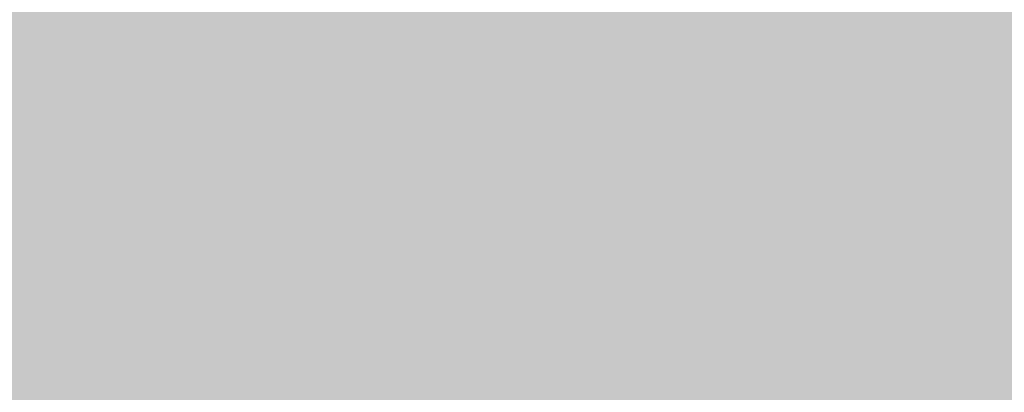
# Model space of a CAD drawing. Units: millimetres. Extents: x 0 to 2267, y 0 to 1823.
# Tile 47 of 256: x 1594.2193 to 1595.0978, y 1226.3857 to 1226.718. Entities that reach past the tile are written whole.
import ezdxf

# ---------------------------------------------------------------- set-up
doc = ezdxf.new("R2010")
doc.units = ezdxf.units.MM
doc.header["$MEASUREMENT"] = 0
doc.layers.add('M-HATC', color=252, linetype='Continuous', lineweight=18)

msp = doc.modelspace()

# ---------------------------------------------------------------- hatches: boundary and pattern name
at = {"layer": 'M-HATC'}
h = msp.add_hatch(color=256, dxfattribs=at)
h.dxf.hatch_style = 1
h.paths.add_polyline_path([(2055.77105, 1603.06204), (1381.08677, 1603.06204), (1381.08677, 1598.06204), (2055.77105, 1598.06204)])
h.paths.add_polyline_path([(2055.77105, 1598.06204), (1381.08677, 1598.06204), (1381.08677, 1593.06204), (2055.77105, 1593.06204)])
h.paths.add_polyline_path([(2051.30737, 1536.76088), (1385.55044, 1536.76088), (1385.55044, 1526.76088), (1387.55044, 1526.76088), (1388.53662, 1525.05276), (1385.33187, 1521.23348), (1385.33187, 1521.22256), (2050.25417, 1522.74913), (2048.32119, 1525.05276), (2049.30737, 1526.76088), (2051.30737, 1526.76088)])
edge = h.paths.add_edge_path()
edge.add_arc((1847.53451, 1379.14917), 135, 222.6030607, 222.8908505, ccw=False)
edge.add_line((1748.16629, 1287.76561), (1683.09212, 1287.76561))
edge.add_arc((1583.7239, 1379.14917), 135, 317.1091495, 317.3969393, ccw=False)
edge.add_arc((1678.9686, 1290.67067), 5, 222.89085, 317.10915, ccw=False)
edge.add_arc((1774.21331, 1379.14917), 135, 222.6030607, 222.8908505, ccw=False)
edge.add_line((1674.84509, 1287.76561), (1609.77092, 1287.76561))
edge.add_arc((1510.4027, 1379.14917), 135, 317.1091495, 317.3969393, ccw=False)
edge.add_arc((1605.6474, 1290.67067), 5, 222.89085, 317.10915, ccw=False)
edge.add_arc((1700.89211, 1379.14917), 135, 222.6030607, 222.8908505, ccw=False)
edge.add_line((1601.52388, 1287.76561), (1536.44972, 1287.76561))
edge.add_arc((1437.08149, 1379.14917), 135, 317.1091495, 317.3969393, ccw=False)
edge.add_arc((1532.3262, 1290.67067), 5, 222.89085, 317.10915, ccw=False)
edge.add_arc((1627.57091, 1379.14917), 135, 222.6030607, 222.8908505, ccw=False)
edge.add_line((1528.20268, 1287.76561), (1505.92891, 1287.76561))
edge.add_spline(control_points=[(1505.92891, 1287.76561), (1504.26224, 1287.76561), (1504.26224, 1282.76561), (1505.92891, 1282.76561)], knot_values=[0, 0, 0, 0, 5, 5, 5, 5], degree=3, periodic=0)
edge.add_line((1505.92891, 1282.76561), (1930.92891, 1282.76561))
edge.add_spline(control_points=[(1930.92891, 1282.76561), (1932.59557, 1282.76561), (1932.59557, 1287.76561), (1930.92891, 1287.76561)], knot_values=[0, 0, 0, 0, 5, 5, 5, 5], degree=3, periodic=0)
edge.add_line((1930.92891, 1287.76561), (1903.05573, 1287.76561))
edge.add_arc((1803.6875, 1379.14917), 135, 317.1091495, 317.3969393, ccw=False)
edge.add_arc((1898.93221, 1290.67067), 5, 222.89085, 317.10915, ccw=False)
edge.add_arc((1994.17691, 1379.14917), 135, 222.6030607, 222.8908505, ccw=False)
edge.add_line((1894.80869, 1287.76561), (1829.73452, 1287.76561))
edge.add_arc((1730.3663, 1379.14917), 135, 317.1091495, 317.3969393, ccw=False)
edge.add_arc((1825.61101, 1290.67067), 5, 222.89085, 317.10915, ccw=False)
edge.add_arc((1920.85571, 1379.14917), 135, 222.6030607, 222.8908505, ccw=False)
edge.add_line((1821.48749, 1287.76561), (1756.41332, 1287.76561))
edge.add_arc((1657.0451, 1379.14917), 135, 317.1091495, 317.3969393, ccw=False)
edge.add_arc((1752.28981, 1290.67067), 5, 222.89085, 317.10915, ccw=False)
edge = h.paths.add_edge_path()
edge.add_spline(control_points=[(1843.42891, 1227.24746), (1845.09557, 1227.24746), (1845.09557, 1232.24746), (1843.42891, 1232.24746)], knot_values=[0, 0, 0, 0, 5, 5, 5, 5], degree=3, periodic=0)
edge.add_line((1843.42891, 1232.24746), (1593.42891, 1232.24746))
edge.add_spline(control_points=[(1593.42891, 1232.24746), (1591.76224, 1232.24746), (1591.76224, 1227.24746), (1593.42891, 1227.24746)], knot_values=[0, 0, 0, 0, 5, 5, 5, 5], degree=3, periodic=0)
edge.add_line((1593.42891, 1227.24746), (1843.42891, 1227.24746))
h.paths.add_polyline_path([(1905.92891, 1127.41706), (1530.92891, 1127.41706, 0.414214), (1520.92891, 1117.41706), (1530.92891, 1117.41706), (1915.92891, 1117.41706, 0.414214)])
edge = h.paths.add_edge_path()
edge.add_arc((1397.08577, 1498.40775), 12.72993, 90.782146, 190.878706, ccw=False)
edge.add_line((1396.912, 1511.13649), (1428.00968, 1511.34875))
edge.add_line((1428.00968, 1511.34875), (1433.00968, 1511.34875))
edge.add_line((1433.00968, 1511.34875), (1434.439, 1511.34875))
edge.add_arc((1419.474, 1498.08041), 20, 41.560995, 74.082109)
edge.add_line((1424.95919, 1517.31353), (1399.93509, 1517.25608))
edge.add_spline(control_points=[(1399.93074, 1517.25607), (1399.88398, 1517.21312), (1399.8328, 1517.16893), (1399.77741, 1517.1236)], knot_values=[11.567499, 11.567499, 11.567499, 11.567499, 11.814249, 11.814249, 11.814249, 11.814249], degree=3, periodic=0)
edge.add_spline(control_points=[(1399.63279, 1517.00986), (1399.58305, 1516.97214), (1399.53072, 1516.93375), (1399.47591, 1516.89474)], knot_values=[11.167718, 11.167718, 11.167718, 11.167718, 11.365188, 11.365188, 11.365188, 11.365188], degree=3, periodic=0)
edge.add_spline(control_points=[(1399.33981, 1516.80007), (1399.15144, 1516.67185), (1398.93836, 1516.5377), (1398.70404, 1516.39942)], knot_values=[10.376405, 10.376405, 10.376405, 10.376405, 11.00994, 11.00994, 11.00994, 11.00994], degree=3, periodic=0)
edge.add_spline(control_points=[(1398.65716, 1516.37187), (1398.57885, 1516.32602), (1398.49825, 1516.27974), (1398.41549, 1516.23309)], knot_values=[10.125175, 10.125175, 10.125175, 10.125175, 10.334406, 10.334406, 10.334406, 10.334406], degree=3, periodic=0)
edge.add_spline(control_points=[(1398.26422, 1516.14874), (1398.19595, 1516.11107), (1398.12634, 1516.07319), (1398.05546, 1516.03513)], knot_values=[9.832246, 9.832246, 9.832246, 9.832246, 9.999658, 9.999658, 9.999658, 9.999658], degree=3, periodic=0)
edge.add_spline(control_points=[(1397.9987, 1516.00476), (1397.73115, 1515.86211), (1397.44602, 1515.71707), (1397.14664, 1515.57138)], knot_values=[9.161808, 9.161808, 9.161808, 9.161808, 9.787769, 9.787769, 9.787769, 9.787769], degree=3, periodic=0)
edge.add_spline(control_points=[(1397.14664, 1515.57138), (1396.84182, 1515.42305), (1396.52223, 1515.27404), (1396.1914, 1515.12621)], knot_values=[8.524455, 8.524455, 8.524455, 8.524455, 9.161808, 9.161808, 9.161808, 9.161808], degree=3, periodic=0)
edge.add_spline(control_points=[(1396.07771, 1515.07565), (1395.98538, 1515.03478), (1395.89222, 1514.99402), (1395.7983, 1514.9534)], knot_values=[8.275193, 8.275193, 8.275193, 8.275193, 8.451726, 8.451726, 8.451726, 8.451726], degree=3, periodic=0)
edge.add_spline(control_points=[(1395.60184, 1514.86912), (1395.49975, 1514.82568), (1395.39685, 1514.78244), (1395.29322, 1514.73944)], knot_values=[7.962917, 7.962917, 7.962917, 7.962917, 8.152764, 8.152764, 8.152764, 8.152764], degree=3, periodic=0)
edge.add_spline(control_points=[(1395.21158, 1514.70568), (1394.82779, 1514.5475), (1394.43452, 1514.39287), (1394.03645, 1514.24422)], knot_values=[7.21254, 7.21254, 7.21254, 7.21254, 7.913148, 7.913148, 7.913148, 7.913148], degree=3, periodic=0)
edge.add_spline(control_points=[(1394.03645, 1514.24422), (1393.70758, 1514.12142), (1393.37544, 1514.0027), (1393.04267, 1513.88945)], knot_values=[6.633733, 6.633733, 6.633733, 6.633733, 7.21254, 7.21254, 7.21254, 7.21254], degree=3, periodic=0)
edge.add_spline(control_points=[(1392.82142, 1513.81499), (1392.71978, 1513.78118), (1392.61815, 1513.74791), (1392.51658, 1513.71521)], knot_values=[6.328796, 6.328796, 6.328796, 6.328796, 6.505493, 6.505493, 6.505493, 6.505493], degree=3, periodic=0)
edge.add_spline(control_points=[(1392.51658, 1513.71521), (1392.31873, 1513.65151), (1392.12116, 1513.59001), (1391.92441, 1513.53098)], knot_values=[5.984605, 5.984605, 5.984605, 5.984605, 6.328796, 6.328796, 6.328796, 6.328796], degree=3, periodic=0)
edge.add_spline(control_points=[(1391.79155, 1513.49146), (1391.31215, 1513.35011), (1390.83842, 1513.22392), (1390.37844, 1513.11711)], knot_values=[5.066697, 5.066697, 5.066697, 5.066697, 5.907055, 5.907055, 5.907055, 5.907055], degree=3, periodic=0)
edge.add_spline(control_points=[(1390.37844, 1513.11711), (1390.17973, 1513.07097), (1389.98359, 1513.02845), (1389.79067, 1512.98988)], knot_values=[4.70367, 4.70367, 4.70367, 4.70367, 5.066695, 5.066695, 5.066695, 5.066695], degree=3, periodic=0)
edge.add_spline(control_points=[(1389.42203, 1512.92036), (1389.24588, 1512.88922), (1389.0729, 1512.86172), (1388.90364, 1512.83814)], knot_values=[4.130571, 4.130571, 4.130571, 4.130571, 4.469816, 4.469816, 4.469816, 4.469816], degree=3, periodic=0)
edge.add_spline(control_points=[(1388.90364, 1512.83814), (1388.59103, 1512.7946), (1388.29108, 1512.76444), (1388.00714, 1512.74941)], knot_values=[3.504031, 3.504031, 3.504031, 3.504031, 4.130571, 4.130571, 4.130571, 4.130571], degree=3, periodic=0)
edge.add_spline(control_points=[(1387.9356, 1512.74593), (1387.85378, 1512.74231), (1387.77334, 1512.73997), (1387.69435, 1512.73898)], knot_values=[3.268866, 3.268866, 3.268866, 3.268866, 3.451164, 3.451164, 3.451164, 3.451164], degree=3, periodic=0)
edge.add_spline(control_points=[(1387.33512, 1512.74426), (1387.20757, 1512.74991), (1387.08472, 1512.7597), (1386.96699, 1512.77385)], knot_values=[2.670686, 2.670686, 2.670686, 2.670686, 2.984, 2.984, 2.984, 2.984], degree=3, periodic=0)
edge.add_spline(control_points=[(1386.83274, 1512.79225), (1386.82093, 1512.79407), (1386.80917, 1512.79594), (1386.79747, 1512.79787)], knot_values=[2.516981, 2.516981, 2.516981, 2.516981, 2.549528, 2.549528, 2.549528, 2.549528], degree=3, periodic=0)
edge.add_spline(control_points=[(1386.45257, 1512.87348), (1386.42573, 1512.88105), (1386.39931, 1512.88895), (1386.3733, 1512.89719)], knot_values=[2.095869, 2.095869, 2.095869, 2.095869, 2.17941, 2.17941, 2.17941, 2.17941], degree=3, periodic=0)
edge.add_spline(control_points=[(1386.06911, 1513.01889), (1386.06338, 1513.02174), (1386.05768, 1513.02463), (1386.05201, 1513.02753)], knot_values=[1.72453, 1.72453, 1.72453, 1.72453, 1.745933, 1.745933, 1.745933, 1.745933], degree=3, periodic=0)
edge.add_arc((1399.474, 1498.08041), 20, 131.824322, 180)
edge.add_arc((1630.33362, 1505.54843), 250.97076, 181.7051759, 236.427975)
edge.add_arc((1605.33992, 1483.30441), 218.7822, 238.660829, 243.3496099)
edge.add_arc((1647.09105, 1510.35917), 262.89859, 183.1298361, 237.8534422, ccw=False)
h.paths.add_polyline_path([(1406.53685, 1391.96444, 0.149382), (1491.55061, 1296.44177, -0.129517)], flags=17)
edge = h.paths.add_edge_path()
edge.add_arc((2037.38381, 1498.08041), 20, 0, 48.265868)
edge.add_spline(control_points=[(2050.69731, 1513.00525), (2050.65121, 1512.98471), (2050.60338, 1512.96554), (2050.55388, 1512.94771)], knot_values=[1.835652, 1.835652, 1.835652, 1.835652, 2.000781, 2.000781, 2.000781, 2.000781], degree=3, periodic=0)
edge.add_spline(control_points=[(2050.46156, 1512.91661), (2050.479, 1512.9221), (2050.49625, 1512.92774), (2050.51332, 1512.93353)], knot_values=[2.045477, 2.045477, 2.045477, 2.045477, 2.101389, 2.101389, 2.101389, 2.101389], degree=3, periodic=0)
edge.add_spline(control_points=[(2050.12896, 1512.83416), (2050.19843, 1512.84734), (2050.26573, 1512.86233), (2050.33075, 1512.87919)], knot_values=[2.237629, 2.237629, 2.237629, 2.237629, 2.435841, 2.435841, 2.435841, 2.435841], degree=3, periodic=0)
edge.add_spline(control_points=[(2050.09463, 1512.82783), (2050.10613, 1512.82989), (2050.11757, 1512.832), (2050.12896, 1512.83416)], knot_values=[2.435841, 2.435841, 2.435841, 2.435841, 2.468321, 2.468321, 2.468321, 2.468321], degree=3, periodic=0)
edge.add_spline(control_points=[(2049.78433, 1512.78511), (2049.85521, 1512.79219), (2049.92435, 1512.80077), (2049.99166, 1512.81088)], knot_values=[2.563852, 2.563852, 2.563852, 2.563852, 2.748541, 2.748541, 2.748541, 2.748541], degree=3, periodic=0)
edge.add_spline(control_points=[(2049.4052, 1512.76169), (2049.5364, 1512.76526), (2049.66292, 1512.77299), (2049.78433, 1512.78511)], knot_values=[2.748541, 2.748541, 2.748541, 2.748541, 3.064882, 3.064882, 3.064882, 3.064882], degree=3, periodic=0)
edge.add_spline(control_points=[(2049.16976, 1512.75968), (2049.23364, 1512.7591), (2049.29654, 1512.7594), (2049.35844, 1512.7606)], knot_values=[3.102309, 3.102309, 3.102309, 3.102309, 3.2503, 3.2503, 3.2503, 3.2503], degree=3, periodic=0)
edge.add_spline(control_points=[(2048.85727, 1512.76911), (2048.96378, 1512.76378), (2049.068, 1512.76061), (2049.16976, 1512.75968)], knot_values=[3.2503, 3.2503, 3.2503, 3.2503, 3.486069, 3.486069, 3.486069, 3.486069], degree=3, periodic=0)
edge.add_spline(control_points=[(2048.69241, 1512.77892), (2048.3729, 1512.80093), (2048.0345, 1512.84106), (2047.68175, 1512.89697)], knot_values=[3.606429, 3.606429, 3.606429, 3.606429, 4.2989, 4.2989, 4.2989, 4.2989], degree=3, periodic=0)
edge.add_spline(control_points=[(2047.68175, 1512.89697), (2047.5458, 1512.91852), (2047.40772, 1512.94241), (2047.26776, 1512.96851)], knot_values=[4.2989, 4.2989, 4.2989, 4.2989, 4.565769, 4.565769, 4.565769, 4.565769], degree=3, periodic=0)
edge.add_spline(control_points=[(2047.26776, 1512.96851), (2047.14494, 1512.99141), (2047.02067, 1513.01601), (2046.89514, 1513.04223)], knot_values=[4.565769, 4.565769, 4.565769, 4.565769, 4.799971, 4.799971, 4.799971, 4.799971], degree=3, periodic=0)
edge.add_spline(control_points=[(2046.89514, 1513.04223), (2046.52865, 1513.11875), (2046.15135, 1513.20899), (2045.7676, 1513.31068)], knot_values=[4.799971, 4.799971, 4.799971, 4.799971, 5.483718, 5.483718, 5.483718, 5.483718], degree=3, periodic=0)
edge.add_spline(control_points=[(2045.7676, 1513.31068), (2045.3724, 1513.41539), (2044.97036, 1513.53225), (2044.56625, 1513.65876)], knot_values=[5.483718, 5.483718, 5.483718, 5.483718, 6.187866, 6.187866, 6.187866, 6.187866], degree=3, periodic=0)
edge.add_spline(control_points=[(2044.56625, 1513.65876), (2044.41491, 1513.70614), (2044.26329, 1513.75487), (2044.11163, 1513.80482)], knot_values=[6.187866, 6.187866, 6.187866, 6.187866, 6.451551, 6.451551, 6.451551, 6.451551], degree=3, periodic=0)
edge.add_spline(control_points=[(2044.11163, 1513.80482), (2043.99666, 1513.84269), (2043.88167, 1513.88126), (2043.76676, 1513.92048)], knot_values=[6.451551, 6.451551, 6.451551, 6.451551, 6.651434, 6.651434, 6.651434, 6.651434], degree=3, periodic=0)
edge.add_spline(control_points=[(2043.76676, 1513.92048), (2043.37157, 1514.05536), (2042.97738, 1514.19789), (2042.58863, 1514.34575)], knot_values=[6.651434, 6.651434, 6.651434, 6.651434, 7.338879, 7.338879, 7.338879, 7.338879], degree=3, periodic=0)
edge.add_spline(control_points=[(2042.58863, 1514.34575), (2042.16431, 1514.50715), (2041.74647, 1514.67491), (2041.34086, 1514.84603)], knot_values=[7.338879, 7.338879, 7.338879, 7.338879, 8.089209, 8.089209, 8.089209, 8.089209], degree=3, periodic=0)
edge.add_spline(control_points=[(2041.34086, 1514.84603), (2041.1028, 1514.94647), (2040.86896, 1515.04806), (2040.64049, 1515.1502)], knot_values=[8.089209, 8.089209, 8.089209, 8.089209, 8.529587, 8.529587, 8.529587, 8.529587], degree=3, periodic=0)
edge.add_spline(control_points=[(2040.50999, 1515.20887), (2040.08238, 1515.40218), (2039.67475, 1515.59705), (2039.29495, 1515.78939)], knot_values=[8.613818, 8.613818, 8.613818, 8.613818, 9.44571, 9.44571, 9.44571, 9.44571], degree=3, periodic=0)
edge.add_spline(control_points=[(2039.29495, 1515.78939), (2039.0618, 1515.90746), (2038.83914, 1516.02458), (2038.62878, 1516.1398)], knot_values=[9.44571, 9.44571, 9.44571, 9.44571, 9.956404, 9.956404, 9.956404, 9.956404], degree=3, periodic=0)
edge.add_spline(control_points=[(2038.62878, 1516.1398), (2038.51874, 1516.20007), (2038.41207, 1516.25982), (2038.30903, 1516.31891)], knot_values=[9.956404, 9.956404, 9.956404, 9.956404, 10.223542, 10.223542, 10.223542, 10.223542], degree=3, periodic=0)
edge.add_spline(control_points=[(2038.30903, 1516.31891), (2038.21377, 1516.37354), (2038.12161, 1516.42762), (2038.03275, 1516.48102)], knot_values=[10.223542, 10.223542, 10.223542, 10.223542, 10.47051, 10.47051, 10.47051, 10.47051], degree=3, periodic=0)
edge.add_spline(control_points=[(2038.03275, 1516.48102), (2037.78552, 1516.62961), (2037.56388, 1516.77304), (2037.37225, 1516.909)], knot_values=[10.47051, 10.47051, 10.47051, 10.47051, 11.15767, 11.15767, 11.15767, 11.15767], degree=3, periodic=0)
edge.add_spline(control_points=[(2037.37225, 1516.909), (2037.27893, 1516.9752), (2037.19274, 1517.03963), (2037.11417, 1517.10203)], knot_values=[11.15767, 11.15767, 11.15767, 11.15767, 11.49227, 11.49227, 11.49227, 11.49227], degree=3, periodic=0)
edge.add_spline(control_points=[(2036.85638, 1517.32585), (2036.91481, 1517.26923), (2036.98143, 1517.21027), (2037.05573, 1517.14922)], knot_values=[11.577341, 11.577341, 11.577341, 11.577341, 11.91035, 11.91035, 11.91035, 11.91035], degree=3, periodic=0)
edge.add_spline(control_points=[(2036.80739, 1517.37475), (2036.82301, 1517.35865), (2036.83935, 1517.34235), (2036.85638, 1517.32585)], knot_values=[11.91035, 11.91035, 11.91035, 11.91035, 12.007402, 12.007402, 12.007402, 12.007402], degree=3, periodic=0)
edge.add_spline(control_points=[(2036.70167, 1517.494), (2036.71042, 1517.48299), (2036.71958, 1517.47185), (2036.72913, 1517.4606)], knot_values=[12.184155, 12.184155, 12.184155, 12.184155, 12.255409, 12.255409, 12.255409, 12.255409], degree=3, periodic=0)
edge.add_spline(control_points=[(2036.6159, 1517.6205), (2036.61998, 1517.61304), (2036.6243, 1517.6055), (2036.62885, 1517.59789)], knot_values=[12.487913, 12.487913, 12.487913, 12.487913, 12.541035, 12.541035, 12.541035, 12.541035], degree=3, periodic=0)
edge.add_spline(control_points=[(2036.56349, 1517.78599), (2036.56372, 1517.77936), (2036.56423, 1517.77264), (2036.56502, 1517.76582)], knot_values=[12.911761, 12.911761, 12.911761, 12.911761, 12.968286, 12.968286, 12.968286, 12.968286], degree=3, periodic=0)
edge.add_spline(control_points=[(2036.61663, 1517.93042), (2036.61248, 1517.92586), (2036.60857, 1517.92121), (2036.60491, 1517.91648)], knot_values=[13.382527, 13.382527, 13.382527, 13.382527, 13.433791, 13.433791, 13.433791, 13.433791], degree=3, periodic=0)
edge.add_spline(control_points=[(2036.74902, 1518.01695), (2036.73613, 1518.0116), (2036.72393, 1518.00601), (2036.71242, 1518.00018)], knot_values=[13.726299, 13.726299, 13.726299, 13.726299, 13.809928, 13.809928, 13.809928, 13.809928], degree=3, periodic=0)
edge.add_spline(control_points=[(2036.86043, 1518.05285), (2036.83863, 1518.04743), (2036.81809, 1518.04156), (2036.79879, 1518.03526)], knot_values=[13.910887, 13.910887, 13.910887, 13.910887, 14.02153, 14.02153, 14.02153, 14.02153], degree=3, periodic=0)
edge.add_line((2036.96387, 1518.08041), (2032.38381, 1518.08041))
edge.add_line((2032.38381, 1518.08041), (2027.38381, 1518.08041))
edge.add_line((2027.38381, 1518.08041), (2022.38381, 1518.08041))
edge.add_line((2022.38381, 1518.08041), (2017.38381, 1518.08041))
edge.add_arc((2017.38381, 1498.08041), 20, 90, 138.439005)
edge.add_line((2002.41881, 1511.34875), (2003.84813, 1511.34875))
edge.add_line((2003.84813, 1511.34875), (2008.84813, 1511.34875))
edge.add_line((2008.84813, 1511.34875), (2039.77204, 1511.13768))
edge.add_arc((2039.77204, 1498.40775), 12.72993, -10.878706, 90, ccw=False)
edge.add_arc((1789.76676, 1510.35917), 262.89859, 302.1465578, 356.8701639, ccw=False)
edge.add_arc((1831.51789, 1483.30441), 218.7822, 296.6503901, 301.339171)
edge.add_arc((1806.52419, 1505.54843), 250.97076, 303.572025, 358.2948241)
h.paths.add_polyline_path([(2030.32096, 1391.96444, -0.129517), (1945.3072, 1296.44177, 0.149382)], flags=17)
edge = h.paths.add_edge_path()
edge.add_spline(control_points=[(2037.2464, 1518.08209), (2037.28977, 1518.08098), (2037.33555, 1518.08041), (2037.3838, 1518.08041)], knot_values=[0.000012, 0.000012, 0.000012, 0.000012, 0.144754, 0.144754, 0.144754, 0.144754], degree=3, periodic=0)
edge.add_line((2037.33571, 1518.08041), (2037.00963, 1518.08041))
edge.add_spline(control_points=[(2037.00963, 1518.08041), (2036.98217, 1518.07678), (2036.95605, 1518.07266), (2036.93124, 1518.06808)], knot_values=[14.13465, 14.13465, 14.13465, 14.13465, 14.247197, 14.247197, 14.247197, 14.247197], degree=3, periodic=0)
edge.add_spline(control_points=[(2036.93124, 1518.06808), (2036.92764, 1518.06741), (2036.92407, 1518.06674), (2036.92053, 1518.06605)], knot_values=[14.118315, 14.118315, 14.118315, 14.118315, 14.13465, 14.13465, 14.13465, 14.13465], degree=3, periodic=0)
edge.add_spline(control_points=[(2036.92053, 1518.06605), (2036.9118, 1518.06436), (2036.90323, 1518.06262), (2036.89484, 1518.06081)], knot_values=[14.078086, 14.078086, 14.078086, 14.078086, 14.118315, 14.118315, 14.118315, 14.118315], degree=3, periodic=0)
edge.add_spline(control_points=[(2036.89484, 1518.06081), (2036.88304, 1518.05827), (2036.87157, 1518.05562), (2036.86043, 1518.05285)], knot_values=[14.02153, 14.02153, 14.02153, 14.02153, 14.078086, 14.078086, 14.078086, 14.078086], degree=3, periodic=0)
edge.add_spline(control_points=[(2036.86043, 1518.05285), (2036.83863, 1518.04743), (2036.81809, 1518.04156), (2036.79879, 1518.03526)], knot_values=[13.910887, 13.910887, 13.910887, 13.910887, 14.02153, 14.02153, 14.02153, 14.02153], degree=3, periodic=0)
edge.add_spline(control_points=[(2036.79879, 1518.03526), (2036.79809, 1518.03504), (2036.7974, 1518.03481), (2036.79671, 1518.03458)], knot_values=[13.906906, 13.906906, 13.906906, 13.906906, 13.910887, 13.910887, 13.910887, 13.910887], degree=3, periodic=0)
edge.add_spline(control_points=[(2036.79671, 1518.03458), (2036.78819, 1518.03178), (2036.77991, 1518.02888), (2036.77187, 1518.02591)], knot_values=[13.857826, 13.857826, 13.857826, 13.857826, 13.906906, 13.906906, 13.906906, 13.906906], degree=3, periodic=0)
edge.add_spline(control_points=[(2036.77187, 1518.02591), (2036.76402, 1518.023), (2036.75641, 1518.02002), (2036.74902, 1518.01695)], knot_values=[13.809928, 13.809928, 13.809928, 13.809928, 13.857826, 13.857826, 13.857826, 13.857826], degree=3, periodic=0)
edge.add_spline(control_points=[(2036.74902, 1518.01695), (2036.73613, 1518.0116), (2036.72393, 1518.00601), (2036.71242, 1518.00018)], knot_values=[13.726299, 13.726299, 13.726299, 13.726299, 13.809928, 13.809928, 13.809928, 13.809928], degree=3, periodic=0)
edge.add_spline(control_points=[(2036.71242, 1518.00018), (2036.71211, 1518.00002), (2036.71179, 1517.99986), (2036.71147, 1517.99969)], knot_values=[13.723993, 13.723993, 13.723993, 13.723993, 13.726299, 13.726299, 13.726299, 13.726299], degree=3, periodic=0)
edge.add_spline(control_points=[(2036.71147, 1517.99969), (2036.70634, 1517.99708), (2036.70134, 1517.99441), (2036.69648, 1517.9917)], knot_values=[13.686536, 13.686536, 13.686536, 13.686536, 13.723993, 13.723993, 13.723993, 13.723993], degree=3, periodic=0)
edge.add_spline(control_points=[(2036.69648, 1517.9917), (2036.6919, 1517.98914), (2036.68744, 1517.98654), (2036.6831, 1517.9839)], knot_values=[13.651251, 13.651251, 13.651251, 13.651251, 13.686536, 13.686536, 13.686536, 13.686536], degree=3, periodic=0)
edge.add_spline(control_points=[(2036.6831, 1517.9839), (2036.67641, 1517.97983), (2036.67001, 1517.97566), (2036.6639, 1517.97139)], knot_values=[13.596804, 13.596804, 13.596804, 13.596804, 13.651251, 13.651251, 13.651251, 13.651251], degree=3, periodic=0)
edge.add_spline(control_points=[(2036.6639, 1517.97139), (2036.66358, 1517.97117), (2036.66326, 1517.97094), (2036.66294, 1517.97072)], knot_values=[13.593956, 13.593956, 13.593956, 13.593956, 13.596804, 13.596804, 13.596804, 13.596804], degree=3, periodic=0)
edge.add_spline(control_points=[(2036.66294, 1517.97072), (2036.6603, 1517.96886), (2036.65771, 1517.96698), (2036.65518, 1517.96509)], knot_values=[13.570322, 13.570322, 13.570322, 13.570322, 13.593956, 13.593956, 13.593956, 13.593956], degree=3, periodic=0)
edge.add_spline(control_points=[(2036.65518, 1517.96509), (2036.65251, 1517.9631), (2036.64991, 1517.96108), (2036.64737, 1517.95905)], knot_values=[13.545477, 13.545477, 13.545477, 13.545477, 13.570322, 13.570322, 13.570322, 13.570322], degree=3, periodic=0)
edge.add_spline(control_points=[(2036.64737, 1517.95905), (2036.64721, 1517.95892), (2036.64705, 1517.9588), (2036.64689, 1517.95867)], knot_values=[13.543931, 13.543931, 13.543931, 13.543931, 13.545477, 13.545477, 13.545477, 13.545477], degree=3, periodic=0)
edge.add_spline(control_points=[(2036.64689, 1517.95867), (2036.64121, 1517.95411), (2036.63582, 1517.94945), (2036.63073, 1517.94468)], knot_values=[13.488237, 13.488237, 13.488237, 13.488237, 13.543931, 13.543931, 13.543931, 13.543931], degree=3, periodic=0)
edge.add_spline(control_points=[(2036.63073, 1517.94468), (2036.62817, 1517.94229), (2036.62569, 1517.93988), (2036.62329, 1517.93744)], knot_values=[13.460307, 13.460307, 13.460307, 13.460307, 13.488237, 13.488237, 13.488237, 13.488237], degree=3, periodic=0)
edge.add_spline(control_points=[(2036.62329, 1517.93744), (2036.62151, 1517.93564), (2036.61978, 1517.93383), (2036.61809, 1517.932)], knot_values=[13.439712, 13.439712, 13.439712, 13.439712, 13.460307, 13.460307, 13.460307, 13.460307], degree=3, periodic=0)
edge.add_spline(control_points=[(2036.61809, 1517.932), (2036.6176, 1517.93147), (2036.61711, 1517.93095), (2036.61663, 1517.93042)], knot_values=[13.433791, 13.433791, 13.433791, 13.433791, 13.439712, 13.439712, 13.439712, 13.439712], degree=3, periodic=0)
edge.add_spline(control_points=[(2036.61663, 1517.93042), (2036.61248, 1517.92586), (2036.60857, 1517.92121), (2036.60491, 1517.91648)], knot_values=[13.382527, 13.382527, 13.382527, 13.382527, 13.433791, 13.433791, 13.433791, 13.433791], degree=3, periodic=0)
edge.add_spline(control_points=[(2036.60491, 1517.91648), (2036.60258, 1517.91347), (2036.60036, 1517.91044), (2036.59824, 1517.90737)], knot_values=[13.350017, 13.350017, 13.350017, 13.350017, 13.382527, 13.382527, 13.382527, 13.382527], degree=3, periodic=0)
edge.add_spline(control_points=[(2036.59824, 1517.90737), (2036.59718, 1517.90585), (2036.59616, 1517.90433), (2036.59515, 1517.90279)], knot_values=[13.333922, 13.333922, 13.333922, 13.333922, 13.350017, 13.350017, 13.350017, 13.350017], degree=3, periodic=0)
edge.add_spline(control_points=[(2036.59515, 1517.90279), (2036.59452, 1517.90183), (2036.5939, 1517.90086), (2036.59329, 1517.89989)], knot_values=[13.323828, 13.323828, 13.323828, 13.323828, 13.333922, 13.333922, 13.333922, 13.333922], degree=3, periodic=0)
edge.add_spline(control_points=[(2036.59329, 1517.89989), (2036.59049, 1517.89545), (2036.5879, 1517.89094), (2036.5855, 1517.88637)], knot_values=[13.277545, 13.277545, 13.277545, 13.277545, 13.323828, 13.323828, 13.323828, 13.323828], degree=3, periodic=0)
edge.add_spline(control_points=[(2036.5855, 1517.88637), (2036.58355, 1517.88267), (2036.58174, 1517.87892), (2036.58006, 1517.87513)], knot_values=[13.240119, 13.240119, 13.240119, 13.240119, 13.277545, 13.277545, 13.277545, 13.277545], degree=3, periodic=0)
edge.add_spline(control_points=[(2036.58006, 1517.87513), (2036.57952, 1517.87393), (2036.579, 1517.87272), (2036.57849, 1517.87151)], knot_values=[13.228211, 13.228211, 13.228211, 13.228211, 13.240119, 13.240119, 13.240119, 13.240119], degree=3, periodic=0)
edge.add_spline(control_points=[(2036.57849, 1517.87151), (2036.57796, 1517.87023), (2036.57744, 1517.86896), (2036.57693, 1517.86767)], knot_values=[13.215717, 13.215717, 13.215717, 13.215717, 13.228211, 13.228211, 13.228211, 13.228211], degree=3, periodic=0)
edge.add_spline(control_points=[(2036.57693, 1517.86767), (2036.57548, 1517.86399), (2036.57414, 1517.86027), (2036.57293, 1517.85651)], knot_values=[13.179847, 13.179847, 13.179847, 13.179847, 13.215717, 13.215717, 13.215717, 13.215717], degree=3, periodic=0)
edge.add_spline(control_points=[(2036.57293, 1517.85651), (2036.5713, 1517.8515), (2036.56989, 1517.84641), (2036.56868, 1517.84126)], knot_values=[13.132017, 13.132017, 13.132017, 13.132017, 13.179847, 13.179847, 13.179847, 13.179847], degree=3, periodic=0)
edge.add_spline(control_points=[(2036.56868, 1517.84126), (2036.56844, 1517.84023), (2036.56821, 1517.8392), (2036.56798, 1517.83817)], knot_values=[13.122482, 13.122482, 13.122482, 13.122482, 13.132017, 13.132017, 13.132017, 13.132017], degree=3, periodic=0)
edge.add_spline(control_points=[(2036.56798, 1517.83817), (2036.56758, 1517.83634), (2036.56721, 1517.8345), (2036.56687, 1517.83266)], knot_values=[13.105592, 13.105592, 13.105592, 13.105592, 13.122482, 13.122482, 13.122482, 13.122482], degree=3, periodic=0)
edge.add_spline(control_points=[(2036.56687, 1517.83266), (2036.56622, 1517.82921), (2036.56567, 1517.82574), (2036.5652, 1517.82223)], knot_values=[13.074063, 13.074063, 13.074063, 13.074063, 13.105592, 13.105592, 13.105592, 13.105592], degree=3, periodic=0)
edge.add_spline(control_points=[(2036.5652, 1517.82223), (2036.5652, 1517.82223), (2036.5652, 1517.82223), (2036.5652, 1517.82223)], knot_values=[13.074043, 13.074043, 13.074043, 13.074043, 13.074063, 13.074063, 13.074063, 13.074063], degree=3, periodic=0)
edge.add_spline(control_points=[(2036.5652, 1517.82223), (2036.56443, 1517.81643), (2036.5639, 1517.81055), (2036.56361, 1517.8046)], knot_values=[13.021884, 13.021884, 13.021884, 13.021884, 13.074043, 13.074043, 13.074043, 13.074043], degree=3, periodic=0)
edge.add_spline(control_points=[(2036.56361, 1517.8046), (2036.56358, 1517.80401), (2036.56356, 1517.80342), (2036.56353, 1517.80283)], knot_values=[13.01674, 13.01674, 13.01674, 13.01674, 13.021884, 13.021884, 13.021884, 13.021884], degree=3, periodic=0)
edge.add_spline(control_points=[(2036.56353, 1517.80283), (2036.56344, 1517.80051), (2036.56338, 1517.79817), (2036.56336, 1517.79582)], knot_values=[12.996438, 12.996438, 12.996438, 12.996438, 13.01674, 13.01674, 13.01674, 13.01674], degree=3, periodic=0)
edge.add_spline(control_points=[(2036.56336, 1517.79582), (2036.56334, 1517.79257), (2036.56338, 1517.78929), (2036.56349, 1517.78599)], knot_values=[12.968286, 12.968286, 12.968286, 12.968286, 12.996438, 12.996438, 12.996438, 12.996438], degree=3, periodic=0)
edge.add_spline(control_points=[(2036.56349, 1517.78599), (2036.56372, 1517.77936), (2036.56423, 1517.77264), (2036.56502, 1517.76582)], knot_values=[12.911761, 12.911761, 12.911761, 12.911761, 12.968286, 12.968286, 12.968286, 12.968286], degree=3, periodic=0)
edge.add_spline(control_points=[(2036.56502, 1517.76582), (2036.56503, 1517.76573), (2036.56504, 1517.76564), (2036.56505, 1517.76555)], knot_values=[12.911017, 12.911017, 12.911017, 12.911017, 12.911761, 12.911761, 12.911761, 12.911761], degree=3, periodic=0)
edge.add_spline(control_points=[(2036.56505, 1517.76555), (2036.56541, 1517.76245), (2036.56583, 1517.75933), (2036.56631, 1517.75619)], knot_values=[12.88528, 12.88528, 12.88528, 12.88528, 12.911017, 12.911017, 12.911017, 12.911017], degree=3, periodic=0)
edge.add_spline(control_points=[(2036.56631, 1517.75619), (2036.56673, 1517.75341), (2036.5672, 1517.75062), (2036.56771, 1517.74782)], knot_values=[12.862519, 12.862519, 12.862519, 12.862519, 12.88528, 12.88528, 12.88528, 12.88528], degree=3, periodic=0)
edge.add_spline(control_points=[(2036.56771, 1517.74782), (2036.56779, 1517.74737), (2036.56788, 1517.74692), (2036.56796, 1517.74647)], knot_values=[12.858885, 12.858885, 12.858885, 12.858885, 12.862519, 12.862519, 12.862519, 12.862519], degree=3, periodic=0)
edge.add_spline(control_points=[(2036.56796, 1517.74647), (2036.5692, 1517.73986), (2036.57069, 1517.73316), (2036.57243, 1517.72638)], knot_values=[12.8053, 12.8053, 12.8053, 12.8053, 12.858885, 12.858885, 12.858885, 12.858885], degree=3, periodic=0)
edge.add_spline(control_points=[(2036.57243, 1517.72638), (2036.5734, 1517.72257), (2036.57446, 1517.71874), (2036.57559, 1517.71488)], knot_values=[12.775176, 12.775176, 12.775176, 12.775176, 12.8053, 12.8053, 12.8053, 12.8053], degree=3, periodic=0)
edge.add_spline(control_points=[(2036.57559, 1517.71488), (2036.57628, 1517.71252), (2036.577, 1517.71015), (2036.57775, 1517.70778)], knot_values=[12.756759, 12.756759, 12.756759, 12.756759, 12.775176, 12.775176, 12.775176, 12.775176], degree=3, periodic=0)
edge.add_spline(control_points=[(2036.57775, 1517.70778), (2036.57808, 1517.70674), (2036.57841, 1517.7057), (2036.57875, 1517.70466)], knot_values=[12.748742, 12.748742, 12.748742, 12.748742, 12.756759, 12.756759, 12.756759, 12.756759], degree=3, periodic=0)
edge.add_spline(control_points=[(2036.57875, 1517.70466), (2036.58082, 1517.6983), (2036.58309, 1517.69187), (2036.58557, 1517.68537)], knot_values=[12.69959, 12.69959, 12.69959, 12.69959, 12.748742, 12.748742, 12.748742, 12.748742], degree=3, periodic=0)
edge.add_spline(control_points=[(2036.58557, 1517.68537), (2036.58762, 1517.68001), (2036.5898, 1517.6746), (2036.59213, 1517.66916)], knot_values=[12.659038, 12.659038, 12.659038, 12.659038, 12.69959, 12.69959, 12.69959, 12.69959], degree=3, periodic=0)
edge.add_spline(control_points=[(2036.59213, 1517.66916), (2036.59397, 1517.66482), (2036.59591, 1517.66047), (2036.59793, 1517.65608)], knot_values=[12.626806, 12.626806, 12.626806, 12.626806, 12.659038, 12.659038, 12.659038, 12.659038], degree=3, periodic=0)
edge.add_spline(control_points=[(2036.59793, 1517.65608), (2036.59839, 1517.65507), (2036.59886, 1517.65406), (2036.59934, 1517.65305)], knot_values=[12.619394, 12.619394, 12.619394, 12.619394, 12.626806, 12.626806, 12.626806, 12.626806], degree=3, periodic=0)
edge.add_spline(control_points=[(2036.59934, 1517.65305), (2036.60435, 1517.64236), (2036.60987, 1517.63151), (2036.61589, 1517.6205)], knot_values=[12.541039, 12.541039, 12.541039, 12.541039, 12.619394, 12.619394, 12.619394, 12.619394], degree=3, periodic=0)
edge.add_spline(control_points=[(2036.61589, 1517.6205), (2036.61589, 1517.6205), (2036.6159, 1517.6205), (2036.6159, 1517.6205)], knot_values=[12.541035, 12.541035, 12.541035, 12.541035, 12.541039, 12.541039, 12.541039, 12.541039], degree=3, periodic=0)
edge.add_spline(control_points=[(2036.6159, 1517.6205), (2036.61998, 1517.61304), (2036.6243, 1517.6055), (2036.62885, 1517.59789)], knot_values=[12.487913, 12.487913, 12.487913, 12.487913, 12.541035, 12.541035, 12.541035, 12.541035], degree=3, periodic=0)
edge.add_spline(control_points=[(2036.62885, 1517.59789), (2036.63261, 1517.5916), (2036.63653, 1517.58526), (2036.64061, 1517.57888)], knot_values=[12.443982, 12.443982, 12.443982, 12.443982, 12.487913, 12.487913, 12.487913, 12.487913], degree=3, periodic=0)
edge.add_spline(control_points=[(2036.64061, 1517.57888), (2036.64144, 1517.57757), (2036.64228, 1517.57626), (2036.64313, 1517.57495)], knot_values=[12.434996, 12.434996, 12.434996, 12.434996, 12.443982, 12.443982, 12.443982, 12.443982], degree=3, periodic=0)
edge.add_spline(control_points=[(2036.64313, 1517.57495), (2036.65306, 1517.55958), (2036.66389, 1517.54394), (2036.6756, 1517.52803)], knot_values=[12.329647, 12.329647, 12.329647, 12.329647, 12.434996, 12.434996, 12.434996, 12.434996], degree=3, periodic=0)
edge.add_spline(control_points=[(2036.6756, 1517.52803), (2036.68385, 1517.51682), (2036.69254, 1517.50548), (2036.70167, 1517.494)], knot_values=[12.255409, 12.255409, 12.255409, 12.255409, 12.329647, 12.329647, 12.329647, 12.329647], degree=3, periodic=0)
edge.add_spline(control_points=[(2036.70167, 1517.494), (2036.71042, 1517.48299), (2036.71958, 1517.47185), (2036.72913, 1517.4606)], knot_values=[12.184155, 12.184155, 12.184155, 12.184155, 12.255409, 12.255409, 12.255409, 12.255409], degree=3, periodic=0)
edge.add_spline(control_points=[(2036.72913, 1517.4606), (2036.74363, 1517.44352), (2036.75904, 1517.42617), (2036.77534, 1517.40855)], knot_values=[12.075961, 12.075961, 12.075961, 12.075961, 12.184155, 12.184155, 12.184155, 12.184155], degree=3, periodic=0)
edge.add_spline(control_points=[(2036.77534, 1517.40855), (2036.77631, 1517.4075), (2036.77729, 1517.40645), (2036.77827, 1517.40539)], knot_values=[12.069502, 12.069502, 12.069502, 12.069502, 12.075961, 12.075961, 12.075961, 12.075961], degree=3, periodic=0)
edge.add_spline(control_points=[(2036.77827, 1517.40539), (2036.78768, 1517.39526), (2036.79739, 1517.38505), (2036.80739, 1517.37475)], knot_values=[12.007402, 12.007402, 12.007402, 12.007402, 12.069502, 12.069502, 12.069502, 12.069502], degree=3, periodic=0)
edge.add_spline(control_points=[(2036.80739, 1517.37475), (2036.82301, 1517.35865), (2036.83935, 1517.34235), (2036.85638, 1517.32585)], knot_values=[11.91035, 11.91035, 11.91035, 11.91035, 12.007402, 12.007402, 12.007402, 12.007402], degree=3, periodic=0)
edge.add_spline(control_points=[(2036.85638, 1517.32585), (2036.91481, 1517.26923), (2036.98143, 1517.21027), (2037.05573, 1517.14922)], knot_values=[11.577341, 11.577341, 11.577341, 11.577341, 11.91035, 11.91035, 11.91035, 11.91035], degree=3, periodic=0)
edge.add_spline(control_points=[(2037.05573, 1517.14922), (2037.07471, 1517.13362), (2037.0942, 1517.11789), (2037.11417, 1517.10203)], knot_values=[11.49227, 11.49227, 11.49227, 11.49227, 11.577341, 11.577341, 11.577341, 11.577341], degree=3, periodic=0)
edge.add_spline(control_points=[(2037.11417, 1517.10203), (2037.19274, 1517.03963), (2037.27893, 1516.9752), (2037.37225, 1516.909)], knot_values=[11.15767, 11.15767, 11.15767, 11.15767, 11.49227, 11.49227, 11.49227, 11.49227], degree=3, periodic=0)
edge.add_spline(control_points=[(2037.37225, 1516.909), (2037.56388, 1516.77304), (2037.78552, 1516.62961), (2038.03275, 1516.48102)], knot_values=[10.47051, 10.47051, 10.47051, 10.47051, 11.15767, 11.15767, 11.15767, 11.15767], degree=3, periodic=0)
edge.add_spline(control_points=[(2038.03275, 1516.48102), (2038.12161, 1516.42762), (2038.21377, 1516.37354), (2038.30903, 1516.31891)], knot_values=[10.223542, 10.223542, 10.223542, 10.223542, 10.47051, 10.47051, 10.47051, 10.47051], degree=3, periodic=0)
edge.add_spline(control_points=[(2038.30903, 1516.31891), (2038.41207, 1516.25982), (2038.51874, 1516.20007), (2038.62878, 1516.1398)], knot_values=[9.956404, 9.956404, 9.956404, 9.956404, 10.223542, 10.223542, 10.223542, 10.223542], degree=3, periodic=0)
edge.add_spline(control_points=[(2038.62878, 1516.1398), (2038.83914, 1516.02458), (2039.0618, 1515.90746), (2039.29495, 1515.78939)], knot_values=[9.44571, 9.44571, 9.44571, 9.44571, 9.956404, 9.956404, 9.956404, 9.956404], degree=3, periodic=0)
edge.add_spline(control_points=[(2039.29495, 1515.78939), (2039.67475, 1515.59705), (2040.08238, 1515.40218), (2040.50999, 1515.20887)], knot_values=[8.613818, 8.613818, 8.613818, 8.613818, 9.44571, 9.44571, 9.44571, 9.44571], degree=3, periodic=0)
edge.add_spline(control_points=[(2040.50999, 1515.20887), (2040.55329, 1515.1893), (2040.59679, 1515.16974), (2040.64049, 1515.1502)], knot_values=[8.529587, 8.529587, 8.529587, 8.529587, 8.613818, 8.613818, 8.613818, 8.613818], degree=3, periodic=0)
edge.add_spline(control_points=[(2040.64049, 1515.1502), (2040.86896, 1515.04806), (2041.1028, 1514.94647), (2041.34086, 1514.84603)], knot_values=[8.089209, 8.089209, 8.089209, 8.089209, 8.529587, 8.529587, 8.529587, 8.529587], degree=3, periodic=0)
edge.add_spline(control_points=[(2041.34086, 1514.84603), (2041.74647, 1514.67491), (2042.16431, 1514.50715), (2042.58863, 1514.34575)], knot_values=[7.338879, 7.338879, 7.338879, 7.338879, 8.089209, 8.089209, 8.089209, 8.089209], degree=3, periodic=0)
edge.add_spline(control_points=[(2042.58863, 1514.34575), (2042.97738, 1514.19789), (2043.37157, 1514.05536), (2043.76676, 1513.92048)], knot_values=[6.651434, 6.651434, 6.651434, 6.651434, 7.338879, 7.338879, 7.338879, 7.338879], degree=3, periodic=0)
edge.add_spline(control_points=[(2043.76676, 1513.92048), (2043.88167, 1513.88126), (2043.99666, 1513.84269), (2044.11163, 1513.80482)], knot_values=[6.451551, 6.451551, 6.451551, 6.451551, 6.651434, 6.651434, 6.651434, 6.651434], degree=3, periodic=0)
edge.add_spline(control_points=[(2044.11163, 1513.80482), (2044.26329, 1513.75487), (2044.41491, 1513.70614), (2044.56625, 1513.65876)], knot_values=[6.187866, 6.187866, 6.187866, 6.187866, 6.451551, 6.451551, 6.451551, 6.451551], degree=3, periodic=0)
edge.add_spline(control_points=[(2044.56625, 1513.65876), (2044.97036, 1513.53225), (2045.3724, 1513.41539), (2045.7676, 1513.31068)], knot_values=[5.483718, 5.483718, 5.483718, 5.483718, 6.187866, 6.187866, 6.187866, 6.187866], degree=3, periodic=0)
edge.add_spline(control_points=[(2045.7676, 1513.31068), (2046.15135, 1513.20899), (2046.52865, 1513.11875), (2046.89514, 1513.04223)], knot_values=[4.799971, 4.799971, 4.799971, 4.799971, 5.483718, 5.483718, 5.483718, 5.483718], degree=3, periodic=0)
edge.add_spline(control_points=[(2046.89514, 1513.04223), (2047.02067, 1513.01601), (2047.14494, 1512.99141), (2047.26776, 1512.96851)], knot_values=[4.565769, 4.565769, 4.565769, 4.565769, 4.799971, 4.799971, 4.799971, 4.799971], degree=3, periodic=0)
edge.add_spline(control_points=[(2047.26776, 1512.96851), (2047.40772, 1512.94241), (2047.5458, 1512.91852), (2047.68175, 1512.89697)], knot_values=[4.2989, 4.2989, 4.2989, 4.2989, 4.565769, 4.565769, 4.565769, 4.565769], degree=3, periodic=0)
edge.add_spline(control_points=[(2047.68175, 1512.89697), (2048.0345, 1512.84106), (2048.3729, 1512.80093), (2048.69241, 1512.77892)], knot_values=[3.606429, 3.606429, 3.606429, 3.606429, 4.2989, 4.2989, 4.2989, 4.2989], degree=3, periodic=0)
edge.add_spline(control_points=[(2048.69241, 1512.77892), (2048.74794, 1512.7751), (2048.8029, 1512.77182), (2048.85727, 1512.76911)], knot_values=[3.486069, 3.486069, 3.486069, 3.486069, 3.606429, 3.606429, 3.606429, 3.606429], degree=3, periodic=0)
edge.add_spline(control_points=[(2048.85727, 1512.76911), (2048.96378, 1512.76378), (2049.068, 1512.76061), (2049.16976, 1512.75968)], knot_values=[3.2503, 3.2503, 3.2503, 3.2503, 3.486069, 3.486069, 3.486069, 3.486069], degree=3, periodic=0)
edge.add_spline(control_points=[(2049.16976, 1512.75968), (2049.23364, 1512.7591), (2049.29654, 1512.7594), (2049.35844, 1512.7606)], knot_values=[3.102309, 3.102309, 3.102309, 3.102309, 3.2503, 3.2503, 3.2503, 3.2503], degree=3, periodic=0)
edge.add_spline(control_points=[(2049.35844, 1512.7606), (2049.37409, 1512.76091), (2049.38968, 1512.76127), (2049.4052, 1512.76169)], knot_values=[3.064882, 3.064882, 3.064882, 3.064882, 3.102309, 3.102309, 3.102309, 3.102309], degree=3, periodic=0)
edge.add_spline(control_points=[(2049.4052, 1512.76169), (2049.5364, 1512.76526), (2049.66292, 1512.77299), (2049.78433, 1512.78511)], knot_values=[2.748541, 2.748541, 2.748541, 2.748541, 3.064882, 3.064882, 3.064882, 3.064882], degree=3, periodic=0)
edge.add_spline(control_points=[(2049.78433, 1512.78511), (2049.85521, 1512.79219), (2049.92435, 1512.80077), (2049.99166, 1512.81088)], knot_values=[2.563852, 2.563852, 2.563852, 2.563852, 2.748541, 2.748541, 2.748541, 2.748541], degree=3, periodic=0)
edge.add_spline(control_points=[(2049.99166, 1512.81088), (2050.02648, 1512.81612), (2050.0608, 1512.82177), (2050.09463, 1512.82783)], knot_values=[2.468321, 2.468321, 2.468321, 2.468321, 2.563852, 2.563852, 2.563852, 2.563852], degree=3, periodic=0)
edge.add_spline(control_points=[(2050.09463, 1512.82783), (2050.10613, 1512.82989), (2050.11757, 1512.832), (2050.12896, 1512.83416)], knot_values=[2.435841, 2.435841, 2.435841, 2.435841, 2.468321, 2.468321, 2.468321, 2.468321], degree=3, periodic=0)
edge.add_spline(control_points=[(2050.12896, 1512.83416), (2050.19843, 1512.84734), (2050.26573, 1512.86233), (2050.33075, 1512.87919)], knot_values=[2.237629, 2.237629, 2.237629, 2.237629, 2.435841, 2.435841, 2.435841, 2.435841], degree=3, periodic=0)
edge.add_spline(control_points=[(2050.33075, 1512.87919), (2050.37544, 1512.89077), (2050.41906, 1512.90324), (2050.46156, 1512.91661)], knot_values=[2.101389, 2.101389, 2.101389, 2.101389, 2.237629, 2.237629, 2.237629, 2.237629], degree=3, periodic=0)
edge.add_spline(control_points=[(2050.46156, 1512.91661), (2050.479, 1512.9221), (2050.49625, 1512.92774), (2050.51332, 1512.93353)], knot_values=[2.045477, 2.045477, 2.045477, 2.045477, 2.101389, 2.101389, 2.101389, 2.101389], degree=3, periodic=0)
edge.add_spline(control_points=[(2050.51332, 1512.93353), (2050.52696, 1512.93816), (2050.54048, 1512.94288), (2050.55388, 1512.94771)], knot_values=[2.000781, 2.000781, 2.000781, 2.000781, 2.045477, 2.045477, 2.045477, 2.045477], degree=3, periodic=0)
edge.add_spline(control_points=[(2050.55388, 1512.94771), (2050.60338, 1512.96554), (2050.65121, 1512.98471), (2050.69731, 1513.00525)], knot_values=[1.835652, 1.835652, 1.835652, 1.835652, 2.000781, 2.000781, 2.000781, 2.000781], degree=3, periodic=0)
edge.add_arc((2037.38381, 1498.08041), 20, 48.265868, 90.129934)
edge = h.paths.add_edge_path(flags=16)
edge.add_spline(control_points=[(1386.13885, 1512.98591), (1388.91997, 1511.73946), (1398.03873, 1515.51866), (1399.93074, 1517.25607)], knot_values=[1.831046, 1.831046, 1.831046, 1.831046, 11.814249, 11.814249, 11.814249, 11.814249], degree=3, periodic=0)
edge.add_line((1399.93074, 1517.25607), (1393.74348, 1517.24186))
edge.add_arc((1399.474, 1498.08041), 20, 106.650105, 131.817301)
h = msp.add_hatch(color=256, dxfattribs=at)
h.dxf.hatch_style = 1
h.paths.add_polyline_path([(2042.88863, 1580.17963), (2055.77105, 1593.06204), (1381.08677, 1593.06204), (1393.96918, 1580.17963), (1374.08597, 1560.29642), (2062.77184, 1560.29642)])
h.paths.add_polyline_path([(1843.42891, 1201.32971), (1843.42891, 1227.24746), (1593.42891, 1227.24746), (1593.42891, 1201.32971, -0.228274), (1574.59893, 1162.23457), (1530.92891, 1127.41706), (1905.92891, 1127.41706), (1862.25888, 1162.23457, -0.228274)])

doc.saveas('drawing.dxf')
